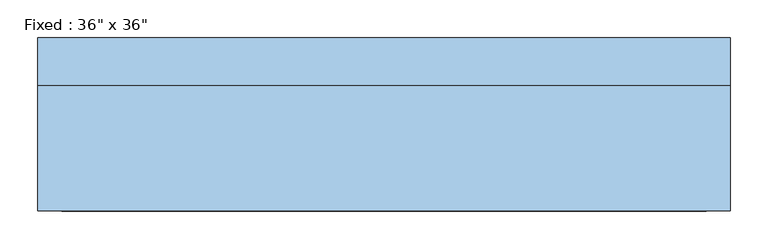
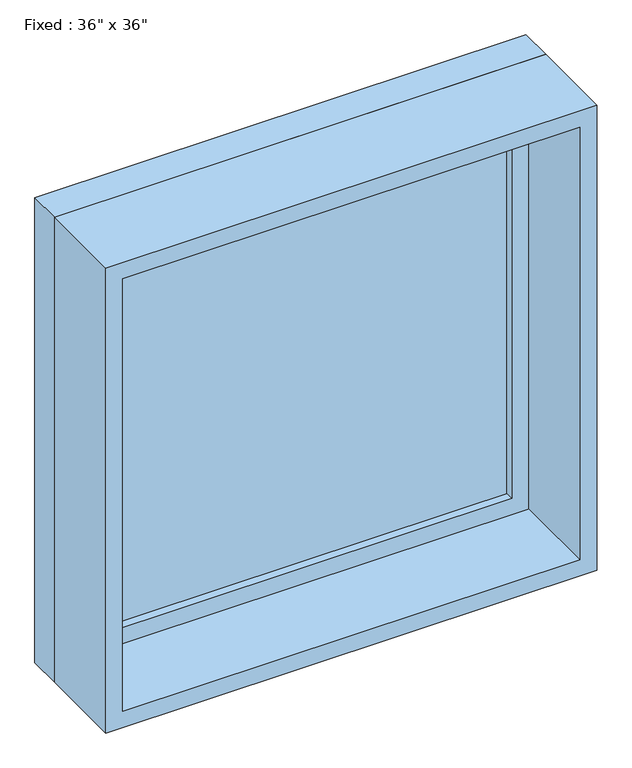
"""IFC4 building model written with IfcOpenShell, lengths in millimetres: window geometry."""

from ifc_helpers import new_model, si_unit, frame, origin, place, context, project, spatial, polyline, outline, extrude, source, transform, mapped, element, save


def window_6c5853a0(model_context):
    return source(origin(), model_context, "Body", "SweptSolid", [
        extrude(outline(polyline([(355.6, 66.675), (-431.8, 66.675), (-431.8, 79.375), (355.6, 79.375), (355.6, 66.675)])), frame((0.0, 0.0, 977.9), z_axis=(0.0, 0.0, 1.0), x_axis=(1.0, 0.0, 0.0)), (0.0, 0.0, 1.0), 787.4),
        extrude(outline(polyline([(1809.75, -476.25), (933.45, -476.25), (933.45, 400.05), (1809.75, 400.05), (1809.75, -476.25)]), holes=[polyline([(1765.3, -431.8), (1765.3, 355.6), (977.9, 355.6), (977.9, -431.8), (1765.3, -431.8)])]), frame((0.0, 50.8, 0.0), z_axis=(0.0, 1.0, 0.0), x_axis=(0.0, 0.0, 1.0)), (0.0, 0.0, 1.0), 44.45),
        extrude(outline(polyline([(1828.8, -495.3), (914.4, -495.3), (914.4, 419.1), (1828.8, 419.1), (1828.8, -495.3)]), holes=[polyline([(1797.05, -463.55), (1797.05, 387.35), (946.15, 387.35), (946.15, -463.55), (1797.05, -463.55)])]), frame((0.0, -114.3, 0.0), z_axis=(0.0, 1.0, 0.0), x_axis=(0.0, 0.0, 1.0)), (0.0, 0.0, 1.0), 165.1),
        extrude(outline(polyline([(1828.8, 419.1), (1828.8, -495.3), (914.4, -495.3), (914.4, 419.1), (1828.8, 419.1)]), holes=[polyline([(1809.75, 400.05), (933.45, 400.05), (933.45, -476.25), (1809.75, -476.25), (1809.75, 400.05)])]), frame((0.0, 50.8, 0.0), z_axis=(0.0, 1.0, 0.0), x_axis=(0.0, 0.0, 1.0)), (0.0, 0.0, 1.0), 63.5),
    ])


if __name__ == "__main__":
    model = new_model("IFC4")
    model_context = context("Model", 3, world=origin())
    ifc_project = project(units=[si_unit("LENGTHUNIT", "METRE", prefix="MILLI")], contexts=[model_context])
    site = spatial("IfcSite", under=ifc_project)
    building = spatial("IfcBuilding", under=site)
    placement = place(None, origin())
    window_shape = window_6c5853a0(model_context)
    element("IfcWindow", 1, ObjectType="Fixed : 36\" x 36\"", at=placement, inside=building, context=model_context, shape_type="MappedRepresentation", body=[
        mapped(window_shape, transform((0.0, 0.0, 0.0), x_axis=(1.0, 0.0, 0.0), y_axis=(0.0, 1.0, 0.0), z_axis=(0.0, 0.0, 1.0))),
    ])
    save(model, "model.ifc")

# Revit data of these elements
# Type "Fixed : 36\" x 36\""
#   Type Mark = "4"
#   Assembly Code = "B2020100"
#   Height = 3' - 0"
#   Default Sill Height = 3' - 0"
#   Width = 3' - 0"
#   Window Inset = 0' - 0 3/4"
#   Glass Pane Material = Glass
#   Sash Material = Sash
#   Wall Closure = (empty or 0)
# Element 1 (IfcWindow, "Fixed : 36\" x 36\"")
#   Materials on its faces: "Sash", "Glass"
# Materials
#   "Glass": class "Glass", colour RGB 218 227 224, transparency 0.85, Description = "Soda Lime Glass", Cost = 0
#   "Sash": class "Wood", colour RGB 136 99 55, transparency 0
